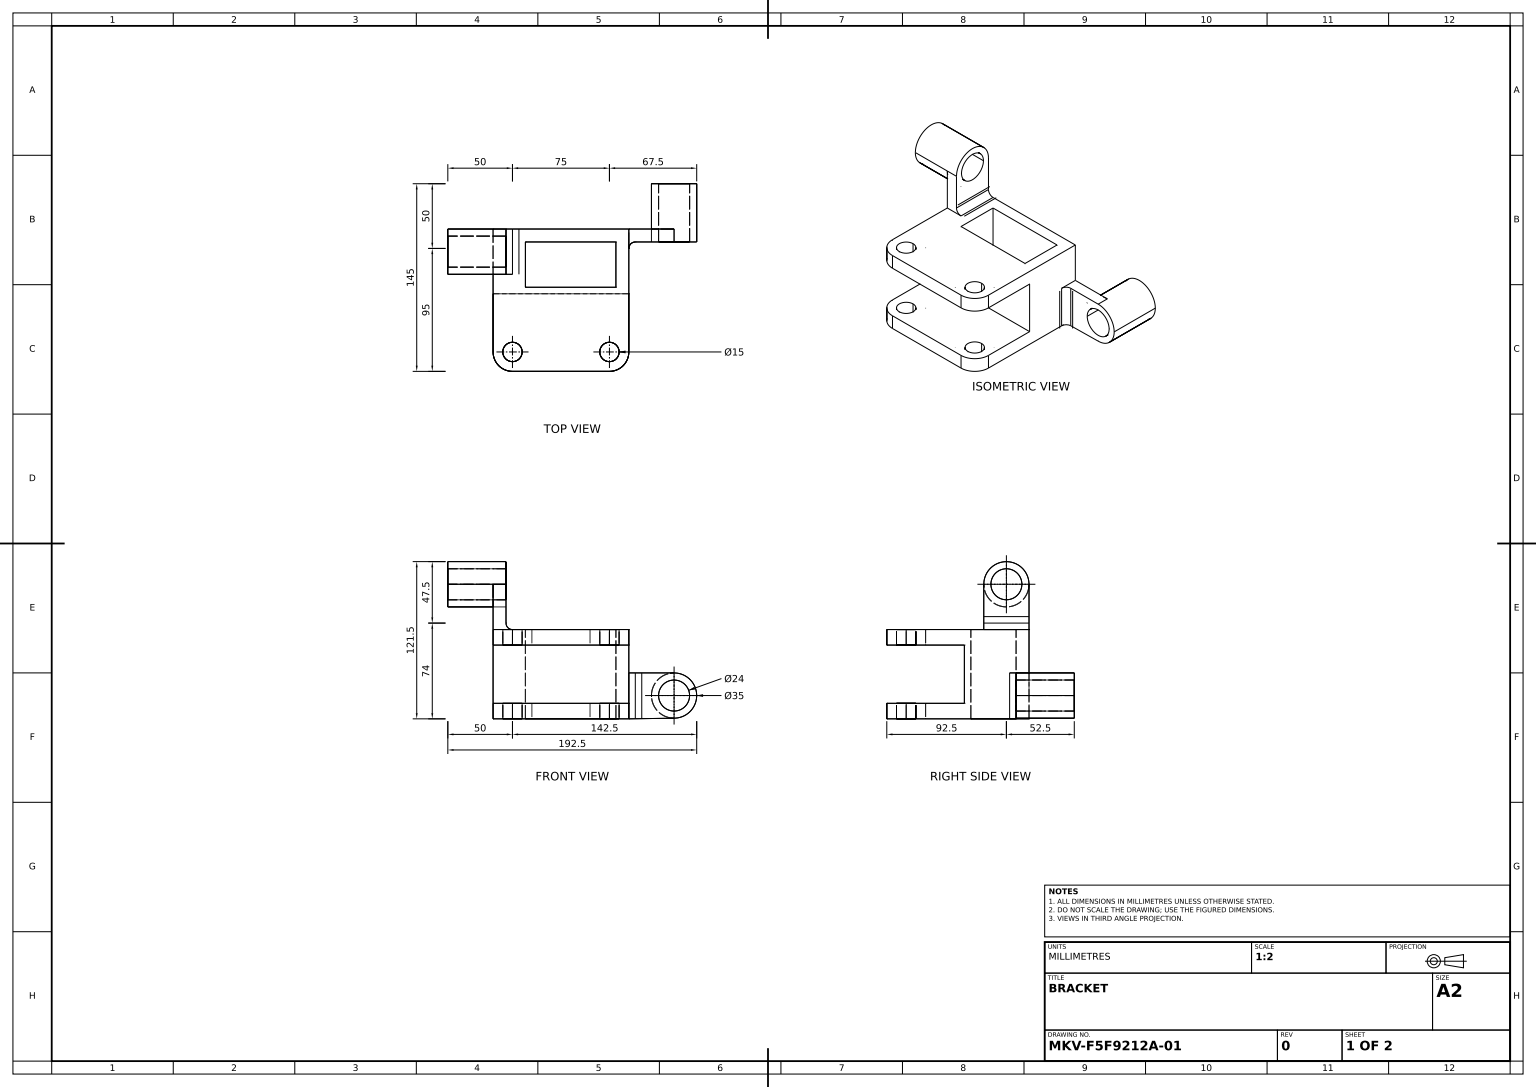
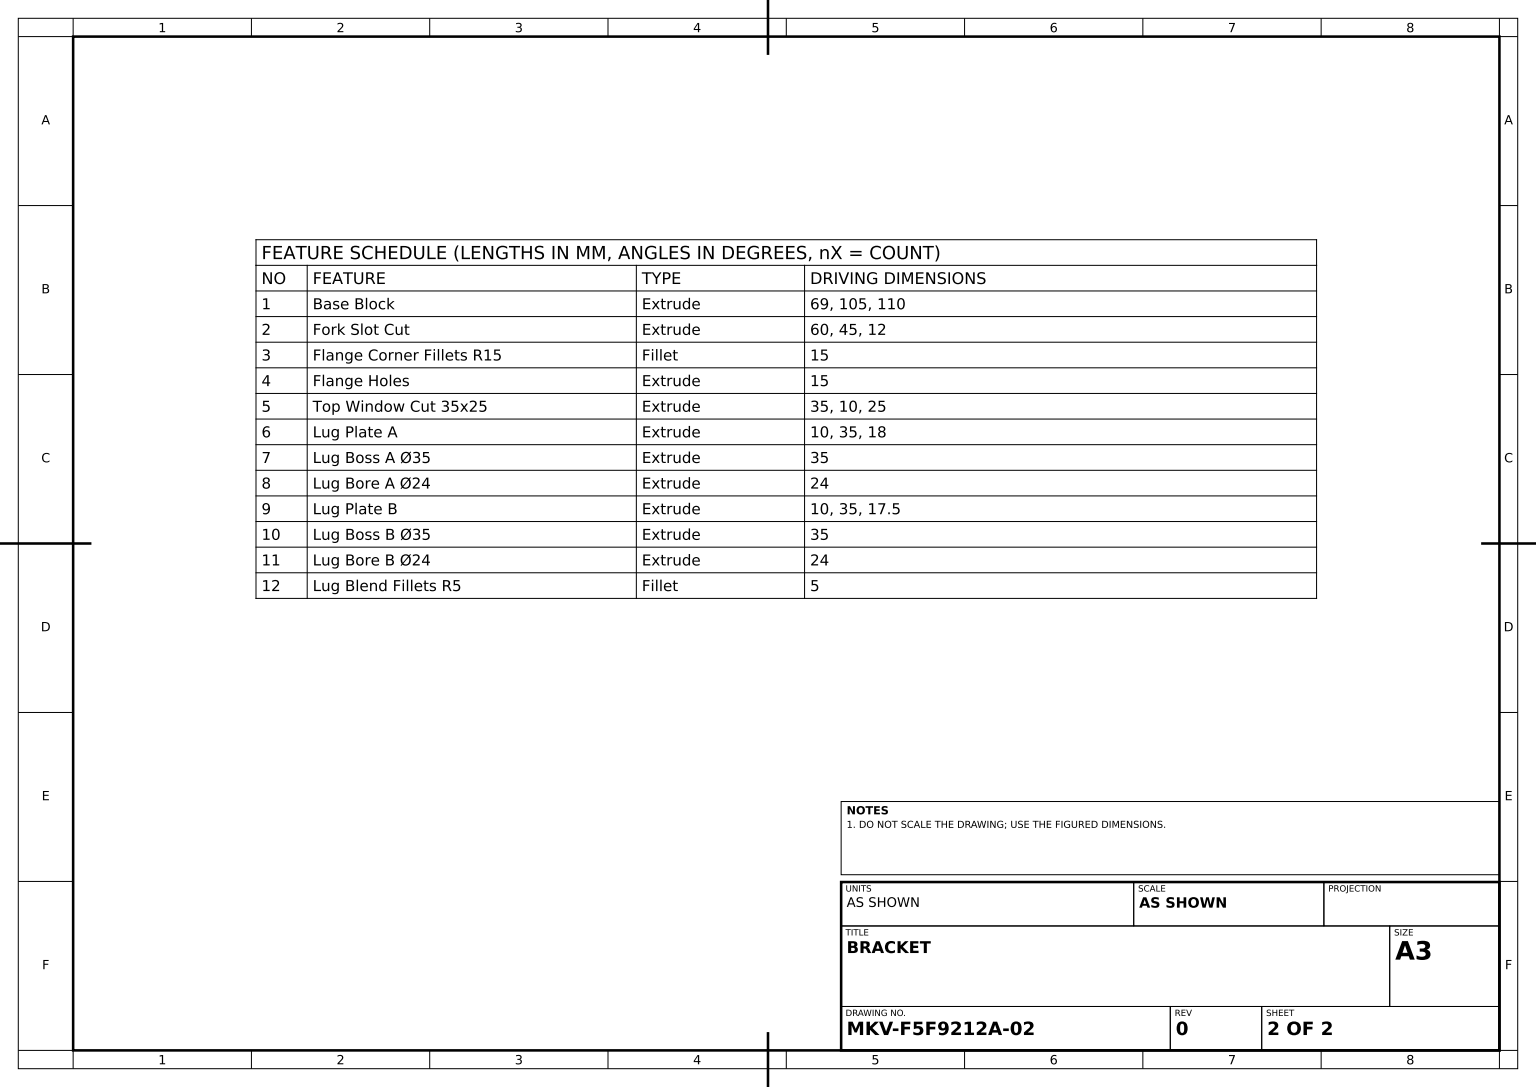
from build123d import *

# Parameters (mm, degrees)
BASE_BLOCK_PROFILE_W        = 105
BASE_BLOCK_PROFILE_H        = 110
BASE_BLOCK_DEPTH            = 69
FORK_SLOT_PROFILE_W         = 105
FORK_SLOT_PROFILE_H         = 45
FORK_SLOT_CUT_DEPTH         = 60
FLANGE_CORNER_FILLETS_R15_R = 15
FLANGE_HOLES_PROFILE_R      = 7.5
FLANGE_HOLES_DEPTH          = 103.67545958
TOP_WINDOW_PROFILE_W        = 70
TOP_WINDOW_PROFILE_H        = 35
TOP_WINDOW_CUT_35X25_DEPTH  = 103.67545958
LUG_PLATE_A_DEPTH           = 10
LUG_START                   = 35
LUG_BOSS_A_PROFILE_R        = 17.5
LUG_BOSS_A_35_DEPTH         = 35
LUG_BORE_A_PROFILE_R        = 12
LUG_BORE_A_24_DEPTH         = 192.861929522
LUG_PLATE_B_DEPTH           = 10
LUG_BOSS_B_PROFILE_R        = 17.5
LUG_BOSS_B_35_DEPTH         = 35
LUG_BORE_B_PROFILE_R        = 12
LUG_BORE_B_24_DEPTH         = 245.782556568
LUG_BLEND_FILLETS_R5_R      = 5


with BuildPart() as part:
    # Base Block Profile → Base Block (new body)
    with BuildSketch(Plane(origin=(0, 0, 0), x_dir=(1, 0, 0), z_dir=(0, 1, 0))):
        Rectangle(BASE_BLOCK_PROFILE_W, BASE_BLOCK_PROFILE_H)
    extrude(amount=BASE_BLOCK_DEPTH)

    # Fork Slot Profile → Fork Slot Cut (cut)
    with BuildSketch(Plane.XY.offset(55)):
        with Locations((0, 34.5)):
            Rectangle(FORK_SLOT_PROFILE_W, FORK_SLOT_PROFILE_H)
    extrude(amount=-FORK_SLOT_CUT_DEPTH, mode=Mode.SUBTRACT)

    # Flange Corner Fillets R15
    flange_corner_fillets_r15_edges = [part.edges().sort_by_distance(p)[0] for p in [
        (52.5, 6, 55),
        (-52.5, 6, 55),
        (52.5, 63, 55),
        (-52.5, 63, 55),
    ]]
    fillet(flange_corner_fillets_r15_edges, radius=FLANGE_CORNER_FILLETS_R15_R)

    # Flange Holes Profile → Flange Holes (cut, through all)
    with BuildSketch(Plane(origin=(0, 69, 0), x_dir=(1, 0, 0), z_dir=(0, 1, 0))):
        with Locations(Location((-37.5, -40, 0), (0, 0, 270))):
            Circle(FLANGE_HOLES_PROFILE_R)
        with Locations(Location((37.5, -40, 0), (0, 0, 270))):
            Circle(FLANGE_HOLES_PROFILE_R)
    extrude(amount=-FLANGE_HOLES_DEPTH, mode=Mode.SUBTRACT)

    # Top Window Profile → Top Window Cut 35x25 (cut, through all)
    with BuildSketch(Plane(origin=(0, 69, 0), x_dir=(1, 0, 0), z_dir=(0, 1, 0))):
        with Locations((7.5, 27.5)):
            Rectangle(TOP_WINDOW_PROFILE_W, TOP_WINDOW_PROFILE_H)
    extrude(amount=-TOP_WINDOW_CUT_35X25_DEPTH, mode=Mode.SUBTRACT)

    # Lug Plate A Profile → Lug Plate A (add)
    with BuildSketch(Plane(origin=(0, 0, -55), x_dir=(-1, 0, 0), z_dir=(0, 0, -1))):
        with BuildLine():
            Line((-87.5, 0.5), (-52.5, 0))
            Line((-52.5, 0), (-52.5, 35.5))
            Line((-52.5, 35.5), (-87.5, 35.5))
            ThreePointArc((-87.5, 35.5), (-105, 18), (-87.5, 0.5))
        make_face()
    extrude(amount=-LUG_PLATE_A_DEPTH)

    # Lug Boss A Profile → Lug Boss A _35 (add)
    with BuildSketch(Plane(origin=(0, 0, -55), x_dir=(-1, 0, 0), z_dir=(0, 0, -1)).offset(LUG_START)):
        with Locations((-87.5, 18)):
            Circle(LUG_BOSS_A_PROFILE_R)
    extrude(amount=-LUG_BOSS_A_35_DEPTH)

    # Lug Bore A Profile → Lug Bore A _24 (cut, through all)
    with BuildSketch(Plane(origin=(0, 0, -90), x_dir=(-1, 0, 0), z_dir=(0, 0, -1))):
        with Locations((-87.5, 18)):
            Circle(LUG_BORE_A_PROFILE_R)
    extrude(amount=-LUG_BORE_A_24_DEPTH, mode=Mode.SUBTRACT)

    # Lug Plate B Profile → Lug Plate B (add)
    with BuildSketch(Plane.ZY.offset(52.5)):
        with BuildLine():
            Line((-55, 104), (-55, 69))
            Line((-55, 69), (-20, 69))
            Line((-20, 69), (-20, 104))
            ThreePointArc((-20, 104), (-37.5, 121.5), (-55, 104))
        make_face()
    extrude(amount=-LUG_PLATE_B_DEPTH)

    # Lug Boss B Profile → Lug Boss B _35 (add)
    with BuildSketch(Plane.ZY.offset(52.5).offset(LUG_START)):
        with Locations((-37.5, 104)):
            Circle(LUG_BOSS_B_PROFILE_R)
    extrude(amount=-LUG_BOSS_B_35_DEPTH)

    # Lug Bore B Profile → Lug Bore B _24 (cut, through all)
    with BuildSketch(Plane.ZY.offset(87.5)):
        with Locations((-37.5, 104)):
            Circle(LUG_BORE_B_PROFILE_R)
    extrude(amount=-LUG_BORE_B_24_DEPTH, mode=Mode.SUBTRACT)

    # Lug Blend Fillets R5
    lug_blend_fillets_r5_edges = [part.edges().sort_by_distance(p)[0] for p in [
        (-42.5, 69, -37.5),
        (52.5, 17.75, -45),
    ]]
    fillet(lug_blend_fillets_r5_edges, radius=LUG_BLEND_FILLETS_R5_R)


solid = part.part
